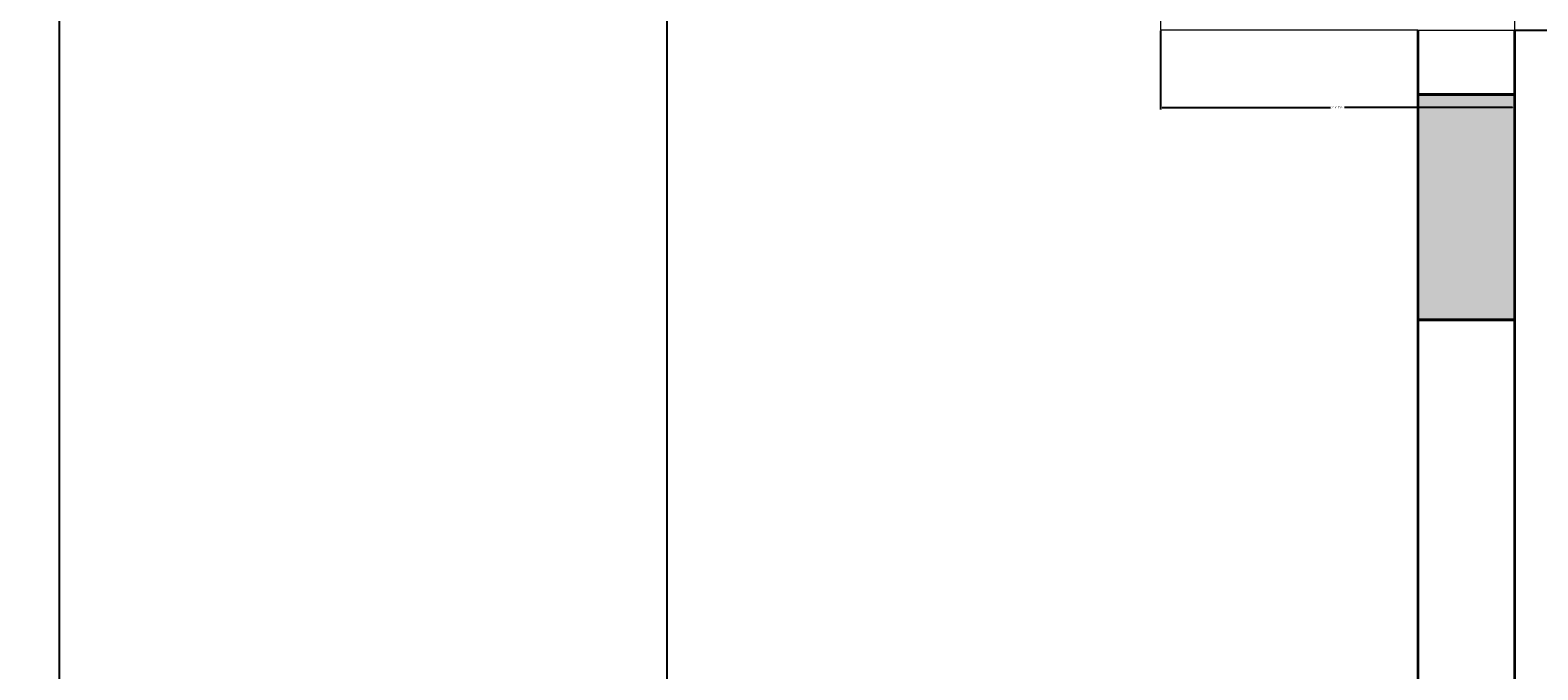
# Model space of a CAD drawing. Units: inches. Extents: x -36 to 401, y -686 to 73.
# Tile 9 of 15: x 184 to 325, y -379 to -319. Entities that reach past the tile are written whole.
import ezdxf

# ---------------------------------------------------------------- set-up
doc = ezdxf.new("R2010")
doc.units = ezdxf.units.IN
doc.header["$MEASUREMENT"] = 0
for name, color, linetype, lineweight in [('A-ANNO-DIMS', 2, 'Continuous', 18), ('A-COLS', 7, 'Continuous', 40), ('A-COLS-PATT', 22, 'Continuous', 13), ('A-DOOR', 3, 'Continuous', 18), ('A-WALL', 7, 'Continuous', 35)]:
    doc.layers.add(name, color=color, linetype=linetype, lineweight=lineweight)
doc.styles.get("Standard").update_dxf_attribs({"font": 'arial.ttf'})
doc.dimstyles.get("Standard").update_dxf_attribs({"dimtxt": 0.18, "dimasz": 0.18, "dimexe": 0.18, "dimexo": 0.0625, "dimgap": 0.09, "dimtad": 0, "dimtih": 1, "dimtoh": 1, "dimdec": 0, "dimzin": 0, "dimdsep": 46, "dimlunit": 3, "dimtxsty": 'Standard', "dimcen": 0.09, "dimadec": 0, "dimazin": 0, "dimtfac": 1, "dimtdec": 0, "dimtofl": 0, "dimtmove": 0, "dimatfit": 3, "dimfxl": 1, "dimtolj": 1, "dimtzin": 0, "dimarcsym": 0})

# ---------------------------------------------------------------- blocks, each defined once
blk = doc.blocks.new('DOOR-PAIR-48IN')
for p, q in [((0, 48), (-24, 48)), ((9, 48), (0, 48)), ((0, 47), (-24, 47)), ((9, 47), (0, 47)), ((0, 1), (-24, 1)), ((0, 0), (-24, 0)), ((0, 1), (9, 1)), ((0, 0), (9, 0))]:
    blk.add_line(p, q)
for centre, start, end in [((1.23, 48), 180, 252.0547), ((1.23, 0), 107.9453, 180)]:
    blk.add_arc(centre, 25.23, start, end)
blk = doc.blocks.new('*D45')
at = {"layer": 'A-ANNO-DIMS', "color": 0, "lineweight": -2, "transparency": 16777216}
for p, q in [((322.75, -271.21), (330.07, -271.21)), ((329.89, -271.39), (329.89, -295.03)), ((329.89, -319.03), (329.89, -295.39)), ((322.75, -319.21), (330.07, -319.21))]:
    blk.add_line(p, q, dxfattribs=at)
at = {"layer": 'A-ANNO-DIMS', "color": 0, "transparency": 16777216}
for points in [[(329.86, -271.39), (329.92, -271.39), (329.89, -271.21)], [(329.86, -319.03), (329.92, -319.03), (329.89, -319.21)]]:
    blk.add_solid(points, dxfattribs=at)
at = {"layer": 'Defpoints', "color": 0, "transparency": 16777216}
for p in [(322.69, -271.21), (329.89, -271.21), (322.69, -319.21)]:
    blk.add_point(p, dxfattribs=at)
at = {"layer": 'A-ANNO-DIMS', "color": 0, "transparency": 16777216, "insert": (329.89, -295.21), "char_height": 0.18, "attachment_point": 5}
blk.add_mtext('\\A1;DOOR PAIR 4\'-0" TYP.', dxfattribs=at)
blk = doc.blocks.new('*D46')
at = {"layer": 'A-ANNO-DIMS', "color": 0, "lineweight": -2, "transparency": 16777216}
for p, q in [((289.69, -319.27), (289.69, -326.59)), ((322.69, -319.27), (322.69, -326.59)), ((289.87, -326.41), (305.55, -326.41)), ((322.51, -326.41), (306.83, -326.41))]:
    blk.add_line(p, q, dxfattribs=at)
at = {"layer": 'A-ANNO-DIMS', "color": 0, "transparency": 16777216}
for points in [[(289.87, -326.38), (289.87, -326.44), (289.69, -326.41)], [(322.51, -326.38), (322.51, -326.44), (322.69, -326.41)]]:
    blk.add_solid(points, dxfattribs=at)
at = {"layer": 'Defpoints', "color": 0, "transparency": 16777216}
for p in [(289.69, -319.21), (322.69, -319.21), (322.69, -326.41)]:
    blk.add_point(p, dxfattribs=at)
at = {"layer": 'A-ANNO-DIMS', "color": 0, "transparency": 16777216, "insert": (306.19, -326.41), "char_height": 0.18, "attachment_point": 5}
blk.add_mtext('\\A1;2\'-9" TYP.', dxfattribs=at)
blk = doc.blocks.new('*D72')
at = {"layer": 'A-ANNO-DIMS', "color": 0, "lineweight": -2, "transparency": 16777216}
for p, q in [((322.75, -319.21), (401.17, -319.21)), ((400.99, -319.39), (400.99, -370.03)), ((400.99, -421.03), (400.99, -370.39)), ((322.75, -421.21), (401.17, -421.21))]:
    blk.add_line(p, q, dxfattribs=at)
at = {"layer": 'A-ANNO-DIMS', "color": 0, "transparency": 16777216}
for points in [[(400.96, -319.39), (401.02, -319.39), (400.99, -319.21)], [(400.96, -421.03), (401.02, -421.03), (400.99, -421.21)]]:
    blk.add_solid(points, dxfattribs=at)
at = {"layer": 'Defpoints', "color": 0, "transparency": 16777216}
for p in [(322.69, -319.21), (322.69, -421.21), (400.99, -421.21)]:
    blk.add_point(p, dxfattribs=at)
at = {"layer": 'A-ANNO-DIMS', "color": 0, "transparency": 16777216, "insert": (400.99, -370.21), "char_height": 0.18, "attachment_point": 5}
blk.add_mtext('\\A1;8\'-6"', dxfattribs=at)
blk = doc.blocks.new('*D87')
at = {"layer": 'A-ANNO-DIMS', "color": 0, "lineweight": -2, "transparency": 16777216}
for p, q in [((243.7, -154.81), (243.7, -685.69)), ((187.11, -163.6), (187.11, -685.69)), ((187.29, -685.51), (214.86, -685.51)), ((243.52, -685.51), (215.95, -685.51))]:
    blk.add_line(p, q, dxfattribs=at)
at = {"layer": 'A-ANNO-DIMS', "color": 0, "transparency": 16777216}
for points in [[(187.29, -685.48), (187.29, -685.54), (187.11, -685.51)], [(243.52, -685.48), (243.52, -685.54), (243.7, -685.51)]]:
    blk.add_solid(points, dxfattribs=at)
at = {"layer": 'Defpoints', "color": 0, "transparency": 16777216}
for p in [(243.7, -154.75), (187.11, -163.53), (243.7, -685.51)]:
    blk.add_point(p, dxfattribs=at)
at = {"layer": 'A-ANNO-DIMS', "color": 0, "transparency": 16777216, "insert": (215.4, -685.51), "char_height": 0.18, "attachment_point": 5}
blk.add_mtext('\\A1;4\'-8 1/2"', dxfattribs=at)

msp = doc.modelspace()

# ---------------------------------------------------------------- hatches: boundary and pattern name
at = {"layer": 'A-COLS-PATT'}
h = msp.add_hatch(color=256, dxfattribs=at)
h.dxf.hatch_style = 1
h.paths.add_polyline_path([(34.69, 7.79), (25.69, 7.79), (25.69, -13.21), (34.69, -13.21)])
h.paths.add_polyline_path([(172.69, -13.21), (177.19, -13.21), (181.69, -13.21), (181.69, 7.79), (172.69, 7.79)])
h.paths.add_polyline_path([(322.69, 7.79), (313.69, 7.79), (313.69, -13.21), (322.69, -13.21)])
h.paths.add_polyline_path([(322.69, -157.21), (313.69, -157.21), (313.69, -178.21), (322.69, -178.21)])
h.paths.add_polyline_path([(172.69, -178.21), (177.19, -178.21), (181.69, -178.21), (181.69, -157.21), (177.19, -157.21), (172.69, -157.21)])
h.paths.add_polyline_path([(25.69, -178.21), (34.69, -178.21), (34.69, -157.21), (25.69, -157.21)])
h.paths.add_polyline_path([(34.69, -325.21), (25.69, -325.21), (25.69, -346.21), (34.69, -346.21)])
h.paths.add_polyline_path([(181.69, -325.21), (177.19, -325.21), (172.69, -325.21), (172.69, -346.21), (177.19, -346.21), (181.69, -346.21)])
h.paths.add_polyline_path([(322.69, -325.21), (313.69, -325.21), (313.69, -346.21), (322.69, -346.21)])
h.paths.add_polyline_path([(364.69, -451.21), (358.69, -451.21), (358.69, -472.21), (364.69, -472.21)])
h.paths.add_polyline_path([(181.69, -451.21), (177.19, -451.21), (172.69, -451.21), (172.69, -472.21), (177.19, -472.21), (181.69, -472.21)])
h.paths.add_polyline_path([(25.69, -472.21), (34.69, -472.21), (34.69, -451.21), (25.69, -451.21)])

# ---------------------------------------------------------------- linework, layer by layer
at = {"layer": 'A-COLS'}
for p, q in [((313.69, -325.21), (322.69, -325.21)), ((313.69, -346.21), (322.69, -346.21))]:
    msp.add_line(p, q, dxfattribs=at)
at = {"layer": 'A-DOOR'}
msp.add_line((322.69, -271.21), (322.69, -319.21), dxfattribs=at)
at = {"layer": 'A-WALL'}
for p, q in [((313.69, -319.21), (313.69, -421.21)), ((322.69, -319.21), (322.69, -421.21))]:
    msp.add_line(p, q, dxfattribs=at)

# ---------------------------------------------------------------- block references
at = {"layer": 'A-DOOR'}
msp.add_blockref('DOOR-PAIR-48IN', (313.69, -319.21), dxfattribs=at)

# ---------------------------------------------------------------- dimensions: what is measured, and where the dimension line sits
at = {"layer": 'A-ANNO-DIMS'}
dim = msp.add_linear_dim(base=(243.7, -685.51), p1=(187.11, -163.53), p2=(243.7, -154.75), dimstyle='Standard', override={"dimdec": 1, "dimlfac": 1, "dimrnd": 0, "dimzin": 1, "dimdsep": 46, "dimlunit": 4, "dimfrac": 2}, dxfattribs=at)
dim.commit()
dim.dimension.update_dxf_attribs({"geometry": '*D87', "text_midpoint": (215.4, -685.51)})
dim = msp.add_linear_dim(base=(329.89, -271.21), p1=(322.69, -319.21), p2=(322.69, -271.21), angle=90, text='DOOR PAIR <> TYP.', dimstyle='Standard', override={"dimdec": 1, "dimlfac": 1, "dimrnd": 0, "dimzin": 1, "dimdsep": 46, "dimlunit": 4, "dimfrac": 2}, dxfattribs=at)
dim.commit()
dim.dimension.update_dxf_attribs({"geometry": '*D45', "text_midpoint": (329.89, -295.21)})
dim = msp.add_linear_dim(base=(322.69, -326.41), p1=(289.69, -319.21), p2=(322.69, -319.21), text='<> TYP.', dimstyle='Standard', override={"dimdec": 1, "dimlfac": 1, "dimrnd": 0, "dimzin": 1, "dimdsep": 46, "dimlunit": 4, "dimfrac": 2}, dxfattribs=at)
dim.commit()
dim.dimension.update_dxf_attribs({"geometry": '*D46', "text_midpoint": (306.19, -326.41)})
dim = msp.add_linear_dim(base=(400.99, -421.21), p1=(322.69, -319.21), p2=(322.69, -421.21), angle=90, dimstyle='Standard', override={"dimdec": 1, "dimlfac": 1, "dimrnd": 0, "dimzin": 1, "dimdsep": 46, "dimlunit": 4, "dimfrac": 2}, dxfattribs=at)
dim.commit()
dim.dimension.update_dxf_attribs({"geometry": '*D72', "text_midpoint": (400.99, -370.21)})

doc.saveas('drawing.dxf')
